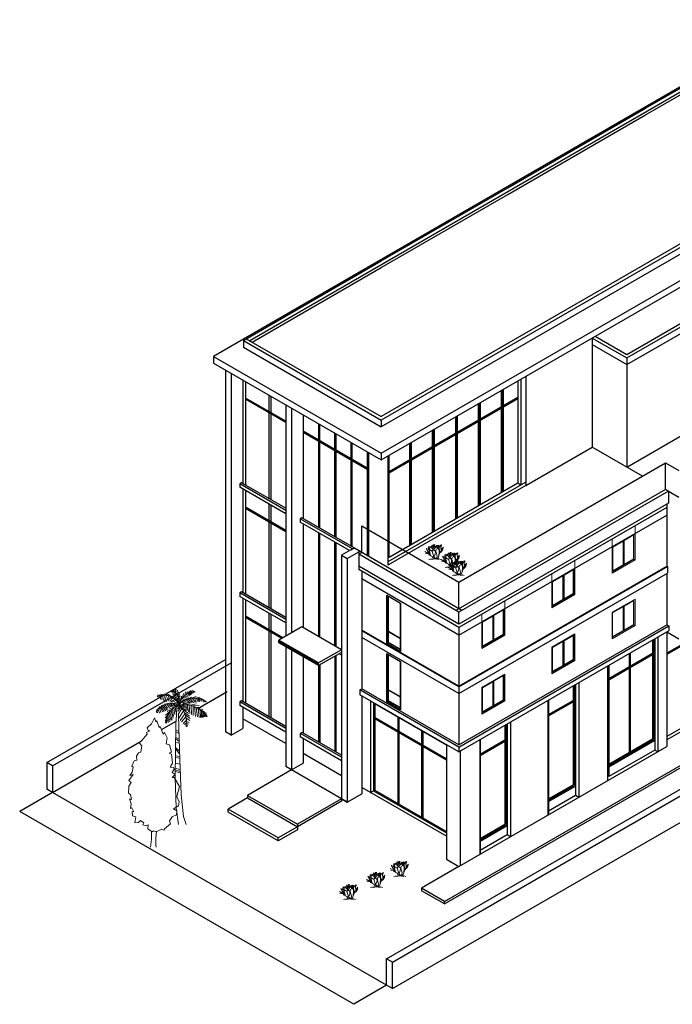
# Model space of a CAD drawing. Units: metres. Extents: x 20738 to 41533, y 14777 to 29586.
# Tile 1 of 2: x 20738 to 20763, y 14777 to 14814. Entities that reach past the tile are written whole.
import ezdxf

# ---------------------------------------------------------------- set-up
doc = ezdxf.new("R2010")
doc.units = ezdxf.units.M
for name, color, linetype, lineweight in [('A-ANNO-NPLT', 8, 'Continuous', 13), ('A-ELEV', 7, 'Continuous', 25), ('A-GLAZ', 4, 'Continuous', 18), ('L-PLNT', 92, 'Continuous', 13)]:
    doc.layers.add(name, color=color, linetype=linetype, lineweight=lineweight)

# ---------------------------------------------------------------- blocks, each defined once
blk = doc.blocks.new('*U2')
for p, q in [((-18.24, 11.04), (-21.755, 16.655)), ((-12.96, 12.48), (-19.68, 16.32)), ((-13.92, 12.48), (-19.2, 14.88)), ((-16.8, 16.32), (-18.72, 18.72)), ((-14.88, 18.24), (-17.76, 19.2)), ((-16.8, 16.32), (-15.36, 19.68)), ((-16.8, 12.48), (-16.8, 16.32)), ((-14.88, 18.24), (-12.96, 20.64)), ((-8.16, 12), (-14.88, 18.24)), ((-13.325, 16.724), (-11.433, 18.289)), ((-12.96, 12.48), (-8.16, 17.76)), ((-12.471, 19.775), (-12.898, 22.044)), ((-11.677, 19.071), (-12.471, 19.775)), ((-11.28, 19.619), (-12.104, 21.184)), ((-12.043, 15.628), (-11.921, 18.836)), ((-11.982, 16.802), (-10.579, 18.054)), ((-11.921, 18.836), (-10.64, 20.401)), ((-11.433, 18.289), (-10.457, 22.749)), ((-10.579, 18.054), (-9.846, 19.697)), ((-8.16, 17.76), (-10.56, 21.6)), ((-9.48, 19.775), (-8.992, 22.592)), ((-7.2, 19.68), (-8.64, 20.16)), ((-8.16, 17.76), (-5.28, 19.2)), ((-7.68, 12.48), (-7.2, 14.88)), ((-7.2, 19.68), (-6.24, 21.12)), ((-4.8, 16.32), (-7.2, 19.68)), ((-7.2, 14.88), (-3.84, 16.8)), ((-5.086, 17.741), (-5.513, 21.34)), ((-5.28, 19.2), (-3.84, 21.6)), ((-3.377, 15.315), (-5.086, 17.819)), ((-2.88, 12.96), (-4.32, 19.68)), ((-3.84, 16.8), (-0.96, 20.64)), ((-3.377, 18.602), (-2.888, 21.575)), ((-2.766, 16.802), (-3.377, 18.602)), ((-2.88, 15.84), (-2.4, 20.16)), ((-0.96, 10.56), (-2.88, 15.84)), ((-0.508, 21.888), (-0.081, 20.558)), ((-0.203, 19.149), (0.102, 21.34)), ((0.346, 13.203), (-0.203, 19.149)), ((-0.142, 19.384), (0.59, 20.401)), ((-0.02, 20.01), (0.896, 21.105)), ((0.041, 20.714), (1.384, 22.044)), ((0.102, 21.34), (0.835, 21.888)), ((0.346, 13.203), (1.323, 16.254)), ((0.96, 12), (1.44, 15.36)), ((0.96, 12), (2.88, 14.88)), ((1.323, 16.254), (3.642, 18.289)), ((1.44, 15.36), (2.88, 17.28)), ((1.92, 13.44), (2.4, 15.36)), ((2.4, 15.36), (3.36, 16.32)), ((-17.76, 8.64), (-23.663, 11.961)), ((-17.76, 8.64), (-23.128, 9.222)), ((-18.24, 11.04), (-20.16, 11.52)), ((-15.84, 8.16), (-18.24, 11.04)), ((-16.32, 7.2), (-18.24, 7.2)), ((-16.8, 12.48), (-17.76, 12.96)), ((-14.88, 5.76), (-17.76, 8.64)), ((-15.84, 0.48), (-17.76, 0)), ((-15.84, 8.16), (-16.8, 12.48)), ((-14.88, 5.76), (-15.84, 8.16)), ((-13.44, 0.48), (-15.84, 0.48)), ((-12.96, 4.8), (-14.88, 5.76)), ((-12.96, 12.48), (-13.92, 12.48)), ((-9.6, 0.96), (-13.44, 0.48)), ((-10.56, 4.32), (-12.96, 12.48)), ((-11.52, 2.4), (-12.96, 4.8)), ((-9.6, 0.96), (-12.96, 0)), ((-8.64, 0.96), (-11.52, 2.4)), ((-10.56, 4.32), (-8.64, 7.68)), ((-8.64, 1.92), (-10.56, 4.32)), ((-9.6, 0.96), (-7.68, 0.96)), ((-8.64, 7.68), (-8.16, 12)), ((-8.64, 0.96), (-4.32, 2.88)), ((-8.64, 0.96), (-6.24, 2.88)), ((-8.64, 0.96), (-8.64, 1.92)), ((-8.64, 0.96), (-2.88, 0.96)), ((-6.72, 8.64), (-7.68, 12.48)), ((-7.68, 0.96), (-6.24, 0.48)), ((-5.76, 5.28), (-6.72, 8.64)), ((-6.24, 2.88), (-5.76, 5.28)), ((-6.24, 0.48), (-3.36, 0)), ((-4.32, 2.88), (-1.92, 9.6)), ((-3.36, 5.28), (-2.88, 12.96)), ((-2.88, 0.96), (0, 0)), ((-1.92, 9.6), (0.96, 12)), ((-0.48, 10.8), (0.346, 13.203))]:
    blk.add_line(p, q)
blk = doc.blocks.new('*U3')
blk.add_lwpolyline([(-2.754, 191.699), (-6.78, 182.851), (-13.682, 176.953), (-11.956, 173.266), (-9.656, 172.529), (-14.257, 170.317), (-13.682, 167.368), (-21.733, 157.783), (-25.184, 154.834), (-21.158, 150.41), (-21.733, 147.461), (-22.884, 140.825), (-26.334, 140.087), (-29.21, 134.926), (-28.635, 129.028), (-32.661, 128.291), (-36.111, 120.18), (-34.386, 118.706), (-35.536, 111.333), (-38.987, 106.171), (-34.386, 107.646), (-40.712, 98.798), (-37.261, 95.849), (-40.712, 90.688), (-41.287, 80.366), (-38.412, 78.154), (-36.686, 70.781), (-39.562, 71.518), (-37.261, 64.145), (-38.412, 57.509), (-36.111, 58.247), (-33.236, 52.348), (-35.536, 53.086), (-34.961, 46.45), (-30.36, 44.975), (-31.51, 36.128), (-26.334, 36.865), (-23.459, 39.814), (-18.283, 36.128), (-20.008, 33.178), (-14.832, 31.704), (-11.956, 33.178), (-12.531, 27.28), (-6.205, 22.856), (-3.905, 24.331), (0.121, 22.856), (8.173, 26.543), (11.624, 25.068), (12.199, 27.28), (21.4, 34.653), (19.675, 39.077), (23.701, 44.975), (30.027, 47.924), (30.602, 53.823), (25.426, 56.772), (32.903, 61.196), (34.053, 67.094), (30.602, 75.205), (34.628, 89.951), (26.576, 103.222), (23.701, 103.222), (28.302, 107.646), (23.701, 110.595), (26.576, 115.756), (25.426, 117.968), (20.825, 118.706), (24.276, 124.604), (22.551, 137.876), (19.1, 139.35), (22.551, 140.825), (19.675, 151.884), (14.499, 153.359), (16.224, 162.207), (12.199, 170.317), (10.473, 167.368), (5.872, 179.165), (4.147, 177.69), (0.696, 187.275), (-0.454, 185.8)], close=True)
for points in [[(-6.813, 23.669), (-6.813, 11.669), (-8.627, 0)], [(0.387, 23.669), (-0.576, 13.271), (-0.576, 3.686), (0, 0)]]:
    blk.add_lwpolyline(points)
blk = doc.blocks.new('*U4')
for p, q in [((-29.729, 190.759), (-31.469, 191.255)), ((-30.309, 190.512), (-30.695, 189.025)), ((-25.283, 191.751), (-29.342, 192.246)), ((-28.763, 190.759), (-28.763, 188.281)), ((-26.443, 191.503), (-26.636, 186.051)), ((-20.064, 191.751), (-25.863, 193.238)), ((-23.737, 191.751), (-24.51, 185.06)), ((-21.031, 191.998), (-21.804, 183.325)), ((-15.232, 191.255), (-20.644, 193.981)), ((-17.551, 191.503), (-20.451, 181.343)), ((-14.265, 190.759), (-18.131, 182.086)), ((-9.433, 189.025), (-15.618, 193.238)), ((-6.727, 197.202), (-11.366, 197.45)), ((-3.441, 194.477), (-10.013, 195.716)), ((-1.894, 192.494), (-9.24, 193.733)), ((-6.147, 186.299), (-9.24, 190.264)), ((-7.5, 199.68), (-7.5, 197.946)), ((-0.541, 189.52), (-7.307, 192.494)), ((-5.76, 190.016), (0.618, 185.308)), ((-5.567, 196.707), (-4.987, 201.167)), ((-4.407, 195.716), (-3.247, 200.672)), ((-2.474, 193.733), (-1.315, 199.433)), ((-1.121, 190.759), (0.232, 196.955)), ((0.038, 188.281), (1.778, 193.981)), ((1.005, 185.803), (2.358, 190.759)), ((4.098, 185.06), (4.678, 190.512)), ((5.837, 187.786), (7.577, 194.229)), ((8.544, 190.512), (13.763, 189.52)), ((9.317, 191.255), (10.283, 196.955)), ((11.25, 192.494), (15.889, 190.512)), ((11.829, 192.99), (13.182, 197.45)), ((13.956, 194.229), (14.729, 196.955)), ((14.536, 193.981), (17.242, 191.255)), ((15.116, 194.477), (17.822, 198.689)), ((16.082, 194.972), (17.822, 192.494)), ((18.015, 195.716), (20.914, 198.689)), ((18.015, 195.468), (18.981, 192.494)), ((19.368, 196.459), (19.948, 193.733)), ((20.914, 196.459), (21.301, 194.972)), ((21.301, 196.459), (22.847, 198.441)), ((22.074, 196.707), (23.427, 195.716)), ((23.234, 196.707), (23.62, 197.698)), ((-21.031, 177.626), (-24.897, 176.387)), ((-24.317, 175.891), (-18.711, 168.457)), ((-22.191, 176.635), (-16.391, 169.448)), ((-15.618, 179.36), (-20.644, 178.617)), ((-20.064, 177.626), (-15.812, 172.67)), ((-17.358, 178.617), (-13.299, 173.661)), ((-11.753, 189.768), (-15.425, 182.83)), ((-15.038, 179.36), (-10.786, 174.404)), ((-8.08, 188.034), (-12.912, 182.83)), ((-12.332, 180.104), (-9.433, 175.643)), ((-4.987, 185.803), (-10.979, 182.086)), ((-10.206, 180.104), (-8.08, 175.891)), ((-1.701, 176.882), (-8.66, 175.396)), ((-8.273, 180.104), (-6.147, 176.635)), ((-3.247, 183.821), (-8.08, 181.838)), ((-6.34, 179.608), (-4.6, 177.13)), ((-5.76, 188.034), (-1.508, 182.582)), ((-1.315, 181.591), (-5.374, 181.095)), ((-4.021, 179.36), (-2.861, 177.378)), ((-2.668, 185.803), (1.198, 181.343)), ((-2.668, 176.387), (-2.376, 170.594)), ((-0.348, 180.352), (-1.894, 180.104)), ((-0.928, 176.882), (-1.508, 173.909)), ((2.551, 175.891), (-0.928, 171.431)), ((1.585, 177.13), (0.038, 174.652)), ((1.005, 182.582), (2.938, 186.547)), ((1.585, 177.13), (6.61, 176.139)), ((2.938, 182.582), (6.61, 183.821)), ((2.938, 175.891), (8.737, 173.413)), ((4.098, 180.847), (8.35, 179.608)), ((4.871, 186.051), (10.09, 186.547)), ((4.871, 181.591), (8.544, 184.812)), ((5.644, 181.838), (13.569, 178.865)), ((6.224, 178.121), (8.157, 175.148)), ((6.997, 188.529), (12.216, 187.786)), ((7.384, 178.369), (10.476, 179.36)), ((7.77, 183.325), (16.082, 179.856)), ((8.157, 178.121), (10.476, 172.422)), ((9.51, 184.317), (15.502, 188.034)), ((10.476, 177.874), (12.796, 169.696)), ((11.25, 184.812), (17.628, 180.352)), ((11.829, 177.874), (18.015, 179.113)), ((13.182, 177.874), (14.729, 166.97)), ((14.536, 185.803), (19.948, 180.847)), ((15.695, 186.299), (19.368, 188.777)), ((15.889, 177.13), (16.855, 164.492)), ((17.242, 186.547), (23.041, 180.599)), ((18.015, 177.13), (26.133, 179.113)), ((18.981, 175.891), (19.561, 163.005)), ((19.368, 187.29), (26.133, 189.768)), ((20.721, 187.042), (25.167, 181.343)), ((20.914, 175.891), (30.966, 176.635)), ((21.688, 175.396), (22.074, 161.518)), ((23.814, 187.29), (26.907, 181.343)), ((24.78, 187.538), (31.546, 188.777)), ((26.133, 187.29), (29.419, 181.838)), ((28.066, 187.29), (30.966, 182.582)), ((29.806, 186.795), (32.319, 183.078)), ((29.999, 186.795), (33.092, 187.29)), ((32.512, 186.299), (35.218, 186.299)), ((33.479, 186.051), (34.445, 182.83)), ((35.605, 185.556), (37.151, 185.308)), ((35.798, 185.308), (36.958, 181.591)), ((38.118, 184.317), (38.504, 181.838)), ((39.857, 182.83), (40.244, 181.591)), ((-32.628, 167.961), (-33.208, 167.961)), ((-32.628, 167.713), (-32.435, 165.979)), ((-28.956, 172.174), (-32.435, 170.192)), ((-31.082, 169.944), (-32.435, 169.2)), ((-31.662, 168.705), (-31.082, 165.483)), ((-27.409, 173.413), (-30.695, 172.67)), ((-29.922, 170.687), (-27.989, 165.235)), ((-25.09, 175.148), (-28.376, 174.404)), ((-27.989, 172.422), (-26.056, 166.227)), ((-26.829, 173.661), (-23.544, 167.218)), ((-25.476, 174.652), (-21.224, 167.466)), ((-14.265, 164.244), (-19.678, 158.049)), ((-12.139, 167.961), (-19.098, 162.014)), ((-8.466, 171.678), (-16.585, 167.713)), ((-15.618, 160.775), (-12.332, 154.332)), ((-14.265, 163.749), (-10.786, 154.828)), ((-4.214, 175.148), (-14.072, 170.935)), ((-12.719, 166.722), (-9.046, 154.828)), ((-10.979, 168.457), (-7.887, 157.801)), ((-8.853, 170.935), (-7.113, 160.527)), ((-6.92, 172.917), (-5.374, 163.253)), ((-4.6, 174.9), (-4.021, 166.722)), ((3.711, 174.404), (-0.541, 167.961)), ((5.257, 171.926), (-0.155, 163.005)), ((7.384, 168.705), (0.812, 157.553)), ((9.317, 164.244), (2.358, 154.332)), ((4.291, 173.909), (12.216, 168.953)), ((6.417, 170.439), (14.729, 164.492)), ((8.544, 165.979), (16.662, 160.527)), ((10.09, 162.51), (17.435, 157.058)), ((23.814, 174.404), (25.554, 160.279)), ((25.554, 173.661), (33.285, 173.661)), ((26.52, 173.165), (28.066, 159.784)), ((28.839, 172.174), (36.378, 170.687)), ((29.226, 171.926), (30.966, 158.545)), ((30.966, 170.687), (38.891, 167.713)), ((32.126, 169.696), (32.512, 158.545)), ((34.058, 168.705), (34.445, 158.545)), ((35.412, 167.713), (41.404, 164.988)), ((36.378, 166.474), (35.605, 158.792)), ((37.731, 165.235), (36.958, 159.288)), ((37.924, 165.235), (41.404, 163.749)), ((38.504, 164.492), (38.504, 159.536)), ((39.664, 163.253), (42.37, 161.766)), ((39.857, 162.757), (39.857, 160.031)), ((40.824, 161.766), (41.21, 160.031)), ((41.21, 161.518), (42.757, 160.279)), ((-16.005, 160.031), (-19.484, 154.084)), ((-18.131, 153.589), (-19.484, 151.606)), ((-17.938, 152.597), (-16.972, 151.111)), ((-17.358, 155.819), (-14.845, 151.358)), ((-16.585, 158.545), (-13.106, 152.35)), ((10.863, 159.784), (4.484, 152.35)), ((11.829, 155.075), (6.804, 150.119)), ((12.603, 151.111), (8.544, 148.385)), ((12.216, 148.137), (10.09, 147.393)), ((11.443, 157.553), (16.855, 154.332)), ((12.216, 153.093), (16.082, 151.606)), ((12.409, 146.898), (13.763, 146.402)), ((12.603, 149.872), (15.116, 149.128)), ((-4.081, 140.645), (0.753, 138.261)), ((-4.081, 137.547), (0.753, 135.163)), ((12.409, 145.659), (11.056, 145.659)), ((-4.081, 129.205), (1.124, 126.821)), ((-4.081, 127.298), (1.31, 123.246)), ((-4.081, 121.578), (1.31, 120.863)), ((-4.639, 102.273), (1.868, 100.604)), ((-4.453, 112.283), (1.682, 105.133)), ((-4.267, 114.428), (1.682, 108.708)), ((-4.453, 99.651), (2.24, 98.459)), ((-4.453, 91.071), (2.426, 89.641)), ((-4.825, 83.921), (2.612, 81.061)), ((-4.639, 81.299), (2.797, 78.916)), ((-4.639, 78.916), (2.797, 76.771))]:
    blk.add_line(p, q)
for points in [[(-2.363, 170.553), (-3.88, 148.505), (-4.988, 69.634), (-3.325, 24.869), (0, 0)], [(-0.116, 162.848), (0.554, 143.532), (2.217, 96.635), (3.88, 44.054), (7.76, 12.079), (11.64, 0)]]:
    blk.add_lwpolyline(points)
for centre, radius, start, end in [((-21.738, 166.094), 25.899, 27.67115, 112.5305), ((-18.427, 181.448), 19.715, 350.285, 64.11229), ((25.595, 171.567), 25.395, 91.40319, 163.882), ((-9.259, 151.732), 28.386, 68.38311, 147.5322), ((14.394, 148.393), 32.752, 113.7592, 177.4133), ((23.687, 155.341), 32.188, 56.19272, 134.3213), ((5.828, 132.718), 45.639, 35.98777, 95.82273), ((-32.8, 147.923), 45.309, 356.1943, 41.37848)]:
    blk.add_arc(centre, radius, start, end)
blk = doc.blocks.new('WIN-SMALL')
for p, q in [((0, 1), (0.866, 1.5)), ((0.866, 0.5), (0.866, 1.5)), ((0.021, 0.985), (0.411, 1.21)), ((0.411, 0.315), (0.411, 1.21)), ((0.454, 1.235), (0.822, 1.448)), ((0.454, 0.34), (0.454, 1.235)), ((0.8, 0.54), (0.8, 1.435)), ((0.822, 0.525), (0.822, 1.448)), ((0, 1), (0, 0)), ((0.021, 0.985), (0.021, 0.062)), ((0, 0), (0.866, 0.5)), ((0.021, 0.062), (0.822, 0.525)), ((0.454, 0.34), (0.8, 0.54)), ((0.798, 0.538), (0.866, 0.5)), ((0.021, 0.09), (0.411, 0.315))]:
    blk.add_line(p, q)
blk = doc.blocks.new('WIN-SMALL-REVEAL')
for p, q in [((0, 1), (0.866, 1.5)), ((0.866, 1.5), (0.866, 1.784)), ((0.866, 0.5), (0.866, 1.5)), ((0, 1), (0, 1.284)), ((0.022, 0.985), (0.412, 1.21)), ((0.412, 0.315), (0.412, 1.21)), ((0.455, 1.235), (0.823, 1.448)), ((0.455, 0.34), (0.455, 1.235)), ((0.801, 0.54), (0.801, 1.435)), ((0.823, 0.525), (0.823, 1.448)), ((0, 1), (0, 0)), ((0.022, 0.985), (0.022, 0.062)), ((0, 0), (0.866, 0.5)), ((0.022, 0.062), (0.823, 0.525)), ((0.455, 0.34), (0.801, 0.54)), ((0.799, 0.539), (0.866, 0.5)), ((0.022, 0.09), (0.412, 0.315))]:
    blk.add_line(p, q)

msp = doc.modelspace()

# ---------------------------------------------------------------- linework, layer by layer
at = {"layer": 'A-ANNO-NPLT'}
msp.add_point((20751.662, 14784.707), dxfattribs=at)
at = {"layer": 'A-ELEV'}
for p, q in [((20767.197, 14813.979), (20745.234, 14801.298)), ((20746.597, 14801.891), (20767.143, 14813.754)), ((20761.514, 14810.649), (20767.143, 14813.899)), ((20761.514, 14810.399), (20767.143, 14813.649)), ((20772.339, 14810.899), (20751.555, 14798.899)), ((20772.101, 14810.891), (20751.555, 14799.029)), ((20772.339, 14810.649), (20751.555, 14798.649)), ((20756.318, 14807.649), (20761.514, 14810.649)), ((20751.555, 14797.649), (20773.518, 14810.329)), ((20751.555, 14797.399), (20773.518, 14810.079)), ((20756.318, 14807.399), (20761.514, 14810.399)), ((20751.555, 14804.899), (20756.318, 14807.649)), ((20751.555, 14804.649), (20756.318, 14807.399)), ((20746.359, 14801.899), (20751.555, 14804.899)), ((20746.688, 14801.839), (20751.555, 14804.649)), ((20760.804, 14801.239), (20766.867, 14804.739)), ((20760.804, 14801.369), (20766.641, 14804.739)), ((20760.804, 14800.989), (20766.867, 14804.489)), ((20746.359, 14801.899), (20751.555, 14798.899)), ((20746.359, 14801.899), (20746.359, 14801.649)), ((20746.471, 14801.964), (20751.555, 14799.029)), ((20759.505, 14801.989), (20759.505, 14797.881)), ((20759.505, 14801.989), (20760.804, 14801.239)), ((20759.618, 14802.054), (20760.804, 14801.369)), ((20746.359, 14801.649), (20751.555, 14798.649)), ((20759.505, 14801.739), (20760.804, 14800.989)), ((20745.234, 14801.298), (20751.555, 14797.649)), ((20745.234, 14801.298), (20745.234, 14801.048)), ((20760.804, 14801.239), (20760.804, 14797.131)), ((20745.234, 14801.048), (20751.555, 14797.399)), ((20745.688, 14800.786), (20745.688, 14787.16)), ((20745.904, 14800.661), (20745.904, 14787.035)), ((20746.337, 14800.411), (20746.337, 14796.512)), ((20756.808, 14800.432), (20756.808, 14796.453)), ((20756.998, 14800.542), (20756.998, 14796.433)), ((20756.998, 14800.542), (20756.998, 14796.433)), ((20760.804, 14797.131), (20766.733, 14800.554)), ((20746.441, 14800.351), (20746.441, 14796.452)), ((20756.089, 14796.193), (20756.089, 14800.017)), ((20756.111, 14796.181), (20756.111, 14800.029)), ((20756.154, 14796.206), (20756.154, 14800.054)), ((20756.695, 14800.367), (20756.695, 14796.518)), ((20747.961, 14798.853), (20746.441, 14799.73)), ((20747.961, 14798.803), (20746.441, 14799.68)), ((20747.326, 14795.941), (20747.326, 14799.84)), ((20747.413, 14795.891), (20747.413, 14799.79)), ((20756.695, 14799.696), (20751.802, 14796.871)), ((20756.695, 14799.746), (20751.848, 14796.947)), ((20747.961, 14799.474), (20747.961, 14790.764)), ((20748.177, 14799.349), (20748.177, 14790.889)), ((20755.22, 14795.692), (20755.22, 14799.515)), ((20755.241, 14795.679), (20755.241, 14799.527)), ((20755.288, 14795.706), (20755.288, 14799.554)), ((20748.61, 14799.099), (20748.61, 14795.194)), ((20754.362, 14795.196), (20754.362, 14799.019)), ((20754.383, 14795.184), (20754.383, 14799.032)), ((20754.422, 14795.206), (20754.422, 14799.054)), ((20749.198, 14794.854), (20749.198, 14798.759)), ((20749.242, 14794.829), (20749.242, 14798.734)), ((20751.555, 14798.899), (20751.555, 14798.649)), ((20753.556, 14794.706), (20753.556, 14798.554)), ((20751.027, 14797.082), (20748.61, 14798.478)), ((20751.027, 14797.032), (20748.61, 14798.428)), ((20749.808, 14794.502), (20749.808, 14798.407)), ((20749.851, 14794.477), (20749.851, 14798.382)), ((20753.491, 14794.693), (20753.491, 14798.517)), ((20753.513, 14794.681), (20753.513, 14798.529)), ((20750.418, 14794.15), (20750.418, 14798.055)), ((20750.461, 14794.125), (20750.461, 14798.03)), ((20752.625, 14794.193), (20752.625, 14798.017)), ((20752.647, 14794.181), (20752.647, 14798.029)), ((20752.69, 14794.206), (20752.69, 14798.054)), ((20756.998, 14796.433), (20759.505, 14797.881)), ((20760.804, 14797.131), (20759.505, 14797.881)), ((20761.397, 14796.789), (20759.505, 14797.881)), ((20751.027, 14797.703), (20751.027, 14793.792)), ((20751.071, 14797.678), (20751.071, 14793.767)), ((20751.555, 14797.649), (20751.555, 14797.399)), ((20751.802, 14797.542), (20751.802, 14793.433)), ((20751.848, 14793.72), (20751.848, 14797.563)), ((20754.483, 14792.797), (20762.263, 14797.289)), ((20762.263, 14796.289), (20762.263, 14797.289)), ((20762.263, 14797.289), (20762.767, 14796.998)), ((20751.848, 14796.947), (20751.802, 14796.921)), ((20746.291, 14796.538), (20746.225, 14796.5)), ((20747.961, 14795.498), (20746.225, 14796.5)), ((20746.225, 14796.5), (20746.225, 14796.368)), ((20747.961, 14795.366), (20746.225, 14796.368)), ((20747.961, 14795.575), (20746.291, 14796.538)), ((20756.998, 14796.563), (20751.802, 14793.563)), ((20756.998, 14796.433), (20751.802, 14793.433)), ((20756.998, 14796.433), (20751.802, 14793.433)), ((20756.695, 14796.518), (20751.848, 14793.72)), ((20756.808, 14796.453), (20756.695, 14796.518)), ((20746.337, 14796.303), (20746.337, 14792.404)), ((20746.337, 14796.303), (20746.337, 14792.404)), ((20746.441, 14796.243), (20746.441, 14792.344)), ((20746.441, 14796.243), (20746.441, 14792.344)), ((20762.263, 14796.289), (20754.37, 14791.732)), ((20762.376, 14796.224), (20754.483, 14791.667)), ((20756.111, 14796.181), (20756.089, 14796.193)), ((20762.376, 14796.224), (20762.263, 14796.289)), ((20762.376, 14796.224), (20762.376, 14795.772)), ((20762.376, 14796.224), (20762.767, 14795.998)), ((20747.961, 14794.745), (20746.441, 14795.622)), ((20747.961, 14794.695), (20746.441, 14795.572)), ((20747.326, 14791.833), (20747.326, 14795.732)), ((20747.413, 14791.783), (20747.413, 14795.682)), ((20762.376, 14795.772), (20754.483, 14791.215)), ((20762.316, 14795.608), (20754.483, 14791.085)), ((20755.241, 14795.679), (20755.22, 14795.692)), ((20762.316, 14795.738), (20762.316, 14795.323)), ((20748.564, 14795.22), (20748.498, 14795.182)), ((20750.529, 14794.086), (20748.564, 14795.22)), ((20754.383, 14795.184), (20754.362, 14795.196)), ((20754.483, 14790.801), (20762.316, 14795.323)), ((20762.316, 14795.323), (20762.316, 14793.398)), ((20748.498, 14795.182), (20748.498, 14795.055)), ((20750.354, 14793.984), (20748.498, 14795.055)), ((20750.468, 14794.05), (20748.503, 14795.185)), ((20748.61, 14794.991), (20748.61, 14791.086)), ((20748.61, 14794.991), (20748.61, 14791.086)), ((20750.821, 14793.911), (20750.821, 14794.911)), ((20750.821, 14794.911), (20754.483, 14792.797)), ((20749.198, 14790.746), (20749.198, 14794.651)), ((20749.242, 14790.721), (20749.242, 14794.626)), ((20751.972, 14778.485), (20780.169, 14794.764)), ((20753.513, 14794.681), (20753.491, 14794.693)), ((20753.939, 14780.768), (20777.825, 14794.559)), ((20753.939, 14780.673), (20777.825, 14794.463)), ((20749.808, 14790.394), (20749.808, 14794.299)), ((20749.851, 14790.369), (20749.851, 14794.274)), ((20750.412, 14794.017), (20750.529, 14794.086)), ((20754.595, 14791.732), (20750.524, 14794.082)), ((20752.647, 14794.181), (20752.625, 14794.193)), ((20760.684, 14793.431), (20760.684, 14794.381)), ((20750.412, 14794.017), (20750.059, 14793.814)), ((20750.059, 14793.814), (20750.275, 14793.689)), ((20750.059, 14793.814), (20750.059, 14790.179)), ((20750.275, 14793.689), (20750.708, 14793.939)), ((20750.708, 14793.976), (20750.708, 14793.265)), ((20750.708, 14793.846), (20750.821, 14793.911)), ((20754.483, 14791.667), (20750.708, 14793.846)), ((20750.275, 14793.689), (20750.275, 14789.921)), ((20754.483, 14791.215), (20750.708, 14793.395)), ((20751.848, 14793.46), (20751.802, 14793.433)), ((20754.483, 14788.876), (20762.316, 14793.398)), ((20754.483, 14788.851), (20762.338, 14793.386)), ((20762.316, 14793.398), (20762.338, 14793.386)), ((20762.338, 14793.386), (20762.338, 14793.136)), ((20754.483, 14791.085), (20750.708, 14793.265)), ((20750.821, 14793.199), (20750.821, 14788.775)), ((20754.483, 14788.601), (20762.338, 14793.136)), ((20758.418, 14792.123), (20758.418, 14793.073)), ((20767.773, 14793.274), (20762.316, 14790.123)), ((20767.773, 14793.224), (20762.316, 14790.073)), ((20762.316, 14793.123), (20762.316, 14791.183)), ((20754.483, 14790.801), (20750.821, 14792.915)), ((20751.756, 14778.61), (20776.005, 14792.61)), ((20754.483, 14791.797), (20754.483, 14792.797)), ((20746.291, 14792.43), (20746.225, 14792.392)), ((20747.961, 14791.39), (20746.225, 14792.392)), ((20746.225, 14792.392), (20746.225, 14792.259)), ((20747.961, 14791.257), (20746.225, 14792.259)), ((20747.961, 14791.466), (20746.291, 14792.43)), ((20751.766, 14790.488), (20751.766, 14792.308)), ((20751.766, 14792.308), (20752.285, 14792.008)), ((20751.815, 14790.517), (20751.815, 14792.266)), ((20751.827, 14790.524), (20751.827, 14792.273)), ((20746.337, 14792.194), (20746.337, 14788.295)), ((20746.337, 14792.194), (20746.337, 14788.295)), ((20746.441, 14792.134), (20746.441, 14788.235)), ((20746.441, 14792.134), (20746.441, 14788.235)), ((20752.264, 14792.021), (20752.264, 14790.258)), ((20752.285, 14792.008), (20752.285, 14790.188)), ((20760.684, 14790.959), (20760.684, 14791.909)), ((20747.85, 14790.7), (20746.441, 14791.513)), ((20747.326, 14787.724), (20747.326, 14791.624)), ((20747.413, 14787.674), (20747.413, 14791.574)), ((20754.483, 14791.215), (20754.483, 14791.667)), ((20755.776, 14790.598), (20755.776, 14791.548)), ((20747.807, 14790.675), (20746.441, 14791.463)), ((20754.483, 14786.661), (20762.316, 14791.183)), ((20754.483, 14786.582), (20762.385, 14791.144)), ((20762.316, 14791.183), (20762.385, 14791.144)), ((20762.316, 14791.104), (20762.385, 14791.144)), ((20762.385, 14791.144), (20762.385, 14790.963)), ((20748.503, 14791.077), (20747.698, 14790.612)), ((20748.564, 14791.112), (20748.498, 14791.074)), ((20750.059, 14790.249), (20748.564, 14791.112)), ((20754.483, 14788.876), (20750.821, 14790.99)), ((20754.483, 14788.851), (20750.821, 14790.965)), ((20751.827, 14790.942), (20752.264, 14790.69)), ((20751.827, 14790.923), (20752.264, 14790.671)), ((20754.483, 14791.085), (20754.483, 14788.876)), ((20754.483, 14786.401), (20762.316, 14790.923)), ((20762.316, 14790.923), (20762.385, 14790.963)), ((20762.316, 14790.923), (20762.316, 14786.605)), ((20762.316, 14790.923), (20762.767, 14790.663)), ((20749.193, 14789.749), (20747.698, 14790.612)), ((20747.698, 14790.512), (20747.698, 14790.612)), ((20749.193, 14789.699), (20747.698, 14790.562)), ((20749.193, 14789.649), (20747.698, 14790.512)), ((20754.483, 14788.601), (20750.821, 14790.715)), ((20751.766, 14790.488), (20751.827, 14790.524)), ((20752.285, 14790.188), (20751.766, 14790.488)), ((20752.264, 14790.258), (20751.815, 14790.517)), ((20752.264, 14790.272), (20751.827, 14790.524)), ((20758.418, 14789.646), (20758.418, 14790.596)), ((20761.77, 14790.608), (20761.77, 14786.89)), ((20761.814, 14790.633), (20761.814, 14786.865)), ((20761.857, 14790.658), (20761.857, 14786.47)), ((20761.857, 14790.658), (20761.857, 14786.47)), ((20761.969, 14790.723), (20761.969, 14786.405)), ((20747.961, 14790.361), (20747.961, 14785.848)), ((20748.177, 14790.236), (20748.177, 14785.723)), ((20750.059, 14790.249), (20749.193, 14789.749)), ((20750.059, 14790.149), (20749.193, 14789.649)), ((20749.815, 14786.414), (20749.815, 14790.009)), ((20749.859, 14786.389), (20749.859, 14790.034)), ((20750.059, 14790.046), (20749.969, 14790.098)), ((20750.059, 14790.179), (20750.059, 14784.636)), ((20751.766, 14788.288), (20751.766, 14790.108)), ((20751.766, 14790.108), (20752.285, 14789.808)), ((20751.815, 14788.317), (20751.815, 14790.066)), ((20751.827, 14788.324), (20751.827, 14790.073)), ((20760.125, 14789.166), (20761.77, 14790.116)), ((20760.125, 14789.116), (20761.77, 14790.066)), ((20760.903, 14786.389), (20760.903, 14790.108)), ((20760.946, 14786.414), (20760.946, 14790.133)), ((20767.773, 14790.135), (20762.316, 14786.985)), ((20767.773, 14790.005), (20762.316, 14786.855)), ((20738.957, 14785.999), (20745.709, 14789.898)), ((20739.174, 14785.874), (20745.926, 14789.773)), ((20748.61, 14789.986), (20748.61, 14787.11)), ((20749.193, 14789.649), (20749.193, 14789.749)), ((20749.206, 14786.766), (20749.206, 14789.657)), ((20749.249, 14786.741), (20749.249, 14789.682)), ((20750.275, 14789.921), (20750.275, 14784.511)), ((20752.264, 14789.821), (20752.264, 14788.058)), ((20752.285, 14789.808), (20752.285, 14787.988)), ((20760.082, 14789.634), (20760.082, 14785.315)), ((20760.125, 14789.659), (20760.125, 14785.47)), ((20755.776, 14788.123), (20755.776, 14789.073)), ((20758.826, 14788.908), (20758.826, 14785.139)), ((20758.869, 14788.933), (20758.869, 14784.758)), ((20758.994, 14789.005), (20758.994, 14784.687)), ((20744.647, 14788.034), (20745.753, 14788.673)), ((20750.752, 14788.735), (20750.821, 14788.775)), ((20750.752, 14788.735), (20750.752, 14788.555)), ((20754.483, 14786.582), (20750.752, 14788.735)), ((20754.483, 14786.401), (20750.752, 14788.555)), ((20754.483, 14786.661), (20750.821, 14788.775)), ((20751.827, 14788.742), (20752.264, 14788.49)), ((20751.827, 14788.723), (20752.264, 14788.471)), ((20754.483, 14788.851), (20754.483, 14786.661)), ((20758.783, 14788.883), (20758.783, 14785.164)), ((20746.291, 14788.322), (20746.225, 14788.284)), ((20747.961, 14787.282), (20746.225, 14788.284)), ((20746.225, 14788.284), (20746.225, 14788.151)), ((20747.961, 14787.149), (20746.225, 14788.151)), ((20747.961, 14787.358), (20746.291, 14788.322)), ((20750.821, 14788.515), (20750.821, 14784.827)), ((20751.155, 14788.322), (20751.155, 14784.87)), ((20751.268, 14788.257), (20751.268, 14784.935)), ((20751.311, 14788.232), (20751.311, 14784.96)), ((20754.006, 14786.651), (20751.311, 14788.207)), ((20751.766, 14788.288), (20751.827, 14788.324)), ((20752.285, 14787.988), (20751.766, 14788.288)), ((20752.264, 14788.058), (20751.815, 14788.317)), ((20752.264, 14788.072), (20751.827, 14788.324)), ((20757.831, 14788.334), (20757.831, 14784.015)), ((20757.852, 14788.346), (20757.852, 14784.028)), ((20757.852, 14787.804), (20758.783, 14788.341)), ((20757.852, 14787.754), (20758.783, 14788.291)), ((20746.337, 14788.086), (20746.337, 14787.285)), ((20743.273, 14787.241), (20743.823, 14787.559)), ((20747.961, 14786.714), (20746.337, 14787.651)), ((20754.006, 14786.134), (20751.311, 14787.69)), ((20754.006, 14786.084), (20751.311, 14787.64)), ((20752.188, 14784.453), (20752.188, 14787.701)), ((20752.231, 14784.428), (20752.231, 14787.676)), ((20756.257, 14787.425), (20756.257, 14783.656)), ((20756.301, 14787.45), (20756.301, 14783.276)), ((20756.425, 14787.522), (20756.425, 14783.204)), ((20745.904, 14787.035), (20745.688, 14787.16)), ((20745.904, 14787.035), (20746.337, 14787.285)), ((20748.572, 14787.132), (20748.505, 14787.094)), ((20748.505, 14787.094), (20748.505, 14786.967)), ((20750.059, 14786.203), (20748.51, 14787.097)), ((20750.059, 14786.274), (20748.572, 14787.132)), ((20753.086, 14783.935), (20753.086, 14787.182)), ((20753.13, 14783.91), (20753.13, 14787.157)), ((20756.214, 14787.4), (20756.214, 14783.681)), ((20739.174, 14784.874), (20742.489, 14786.789)), ((20750.059, 14786.07), (20748.505, 14786.967)), ((20748.61, 14786.907), (20748.61, 14785.973)), ((20748.62, 14787.034), (20748.618, 14787.035)), ((20755.262, 14786.851), (20755.262, 14782.532)), ((20755.262, 14786.851), (20755.262, 14782.532)), ((20755.284, 14786.863), (20755.284, 14782.545)), ((20755.284, 14786.321), (20756.214, 14786.858)), ((20755.284, 14786.271), (20756.214, 14786.808)), ((20760.125, 14785.94), (20761.77, 14786.89)), ((20760.125, 14785.89), (20761.814, 14786.865)), ((20760.125, 14785.84), (20761.857, 14786.84)), ((20750.059, 14785.503), (20748.61, 14786.339)), ((20754.006, 14786.651), (20754.006, 14782.357)), ((20754.483, 14782.082), (20762.316, 14786.605)), ((20754.483, 14786.582), (20754.483, 14786.401)), ((20754.526, 14786.426), (20754.526, 14782.107)), ((20761.857, 14786.47), (20760.125, 14785.47)), ((20761.969, 14786.405), (20761.857, 14786.47)), ((20738.957, 14785.999), (20738.957, 14784.999)), ((20739.174, 14785.874), (20738.957, 14785.999)), ((20748.177, 14785.723), (20748.61, 14785.973)), ((20739.174, 14785.874), (20739.174, 14784.874)), ((20748.177, 14785.723), (20746.514, 14784.762)), ((20748.177, 14785.723), (20747.961, 14785.848)), ((20750.059, 14784.636), (20748.177, 14785.723)), ((20761.116, 14782.764), (20765.879, 14785.514)), ((20739.174, 14784.874), (20737.933, 14784.158)), ((20739.174, 14784.874), (20738.957, 14784.999)), ((20751.756, 14777.61), (20739.174, 14784.874)), ((20750.275, 14784.511), (20750.821, 14784.827)), ((20754.006, 14783.224), (20750.821, 14785.062)), ((20751.155, 14784.87), (20751.268, 14784.935)), ((20751.268, 14784.935), (20751.311, 14784.96)), ((20751.268, 14784.935), (20754.006, 14783.354)), ((20751.311, 14784.96), (20754.006, 14783.404)), ((20757.852, 14784.627), (20758.783, 14785.164)), ((20757.852, 14784.577), (20758.826, 14785.139)), ((20757.852, 14784.527), (20758.869, 14785.114)), ((20746.514, 14784.665), (20745.783, 14784.244)), ((20746.514, 14784.762), (20748.395, 14783.676)), ((20746.514, 14784.762), (20746.514, 14784.665)), ((20746.514, 14784.665), (20748.395, 14783.579)), ((20750.059, 14784.636), (20748.395, 14783.676)), ((20750.059, 14784.54), (20748.395, 14783.579)), ((20750.059, 14784.636), (20750.275, 14784.511)), ((20750.275, 14784.511), (20750.059, 14784.636)), ((20750.059, 14784.636), (20750.059, 14784.54)), ((20758.869, 14784.758), (20757.852, 14784.171)), ((20758.994, 14784.687), (20758.869, 14784.758)), ((20750.515, 14776.894), (20737.933, 14784.158)), ((20747.665, 14783.158), (20745.783, 14784.244)), ((20745.783, 14784.133), (20745.783, 14784.244)), ((20747.665, 14783.047), (20745.783, 14784.133)), ((20748.395, 14783.579), (20747.665, 14783.158)), ((20748.395, 14783.468), (20747.665, 14783.047)), ((20748.395, 14783.676), (20748.395, 14783.579)), ((20748.395, 14783.579), (20748.395, 14783.468)), ((20755.284, 14783.144), (20756.214, 14783.681)), ((20755.284, 14783.094), (20756.257, 14783.656)), ((20755.284, 14783.044), (20756.301, 14783.631)), ((20747.665, 14783.047), (20747.665, 14783.158)), ((20756.301, 14783.276), (20755.284, 14782.688)), ((20756.425, 14783.204), (20756.301, 14783.276)), ((20751.972, 14777.485), (20761.116, 14782.764)), ((20754.006, 14782.357), (20754.483, 14782.082)), ((20754.483, 14782.082), (20753.073, 14781.268)), ((20753.939, 14780.768), (20753.073, 14781.268)), ((20753.073, 14781.268), (20753.073, 14781.173)), ((20753.939, 14780.673), (20753.073, 14781.173)), ((20753.939, 14780.673), (20753.939, 14780.768)), ((20751.756, 14777.61), (20751.756, 14778.61)), ((20751.972, 14778.485), (20751.756, 14778.61)), ((20751.972, 14777.485), (20751.972, 14778.485)), ((20751.756, 14777.61), (20750.515, 14776.894)), ((20751.972, 14777.485), (20751.756, 14777.61))]:
    msp.add_line(p, q, dxfattribs=at)

# ---------------------------------------------------------------- block references
at = {"layer": 'A-GLAZ'}
for name, p in [('WIN-SMALL-REVEAL', (20760.251, 14793.132)), ('WIN-SMALL-REVEAL', (20757.984, 14791.823)), ('WIN-SMALL-REVEAL', (20755.343, 14790.298)), ('WIN-SMALL', (20760.251, 14790.659)), ('WIN-SMALL', (20757.985, 14789.346)), ('WIN-SMALL', (20755.344, 14787.824))]:
    msp.add_blockref(name, p, dxfattribs=at)
at = {"layer": 'L-PLNT', "xscale": 0.0254, "yscale": 0.0254, "zscale": 0.0254}
for name, p in [('*U2', (20753.803, 14793.643)), ('*U2', (20754.414, 14793.344)), ('*U2', (20754.684, 14793.041)), ('*U4', (20743.913, 14783.663)), ('*U3', (20743.077, 14782.811)), ('*U2', (20752.485, 14781.711)), ('*U2', (20751.602, 14781.293)), ('*U2', (20750.584, 14780.836))]:
    msp.add_blockref(name, p, dxfattribs=at)

doc.saveas('drawing.dxf')
